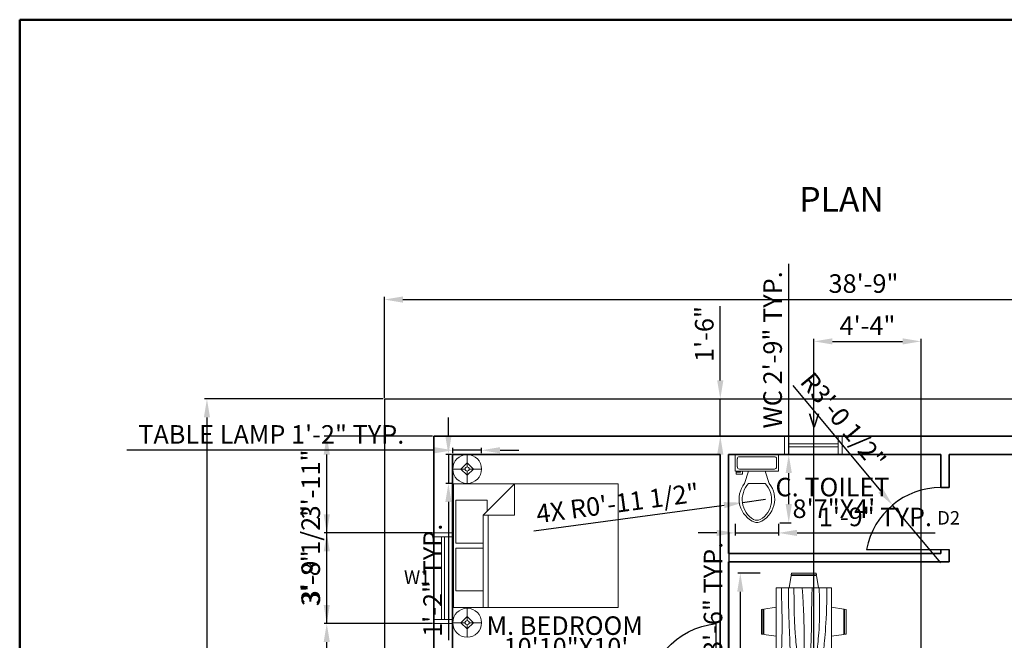
# Model space of a CAD drawing. Units: inches. Extents: x 2113 to 4530, y 1685 to 2353.
# Tile 3 of 6: x 2113 to 2591, y 2052 to 2353. Entities that reach past the tile are written whole.
import ezdxf

# ---------------------------------------------------------------- set-up
doc = ezdxf.new("R2010")
doc.units = ezdxf.units.IN
for name, color, linetype, lineweight in [('A-ANNO-DIMS', 2, 'Continuous', 18), ('A-ANNO-TEXT', 7, 'Continuous', 18), ('A-ANNO-TITL', 7, 'Continuous', 35), ('A-ANNO-TTLB', 7, 'Continuous', 50), ('A-AREA-IDEN', 7, 'Continuous', 18), ('A-DOOR', 3, 'Continuous', 25), ('A-FLOR-FIXT', 9, 'Continuous', 18), ('A-FURN', 8, 'Continuous', 18), ('A-GLAZ', 4, 'Continuous', 18), ('A-WALL', 7, 'Continuous', 35), ('C-PROP', 7, 'Continuous', 25), ('S-ANNO-DIMS', 2, 'Continuous', 18)]:
    doc.layers.add(name, color=color, linetype=linetype, lineweight=lineweight)
doc.styles.get("Standard").update_dxf_attribs({"font": 'arial.ttf'})
doc.dimstyles.new('ISO-25', dxfattribs={"dimtxt": 9, "dimasz": 9, "dimexe": 1.25, "dimexo": 0.625, "dimgap": 2, "dimtad": 1, "dimdec": 1, "dimlunit": 4, "dimtxsty": 'Standard', "dimcen": 2.5, "dimazin": 0, "dimtfac": 1, "dimtdec": 1, "dimtmove": 0, "dimatfit": 3, "dimfxl": 1, "dimarcsym": 0})

# ---------------------------------------------------------------- blocks, each defined once
blk = doc.blocks.new('Dining Set - 36 x 72 in.')
for p, q in [((-22.2343, 26.00059), (-23.4847, 17.99762)), ((-22.2304, 26), (-5.7608, 26)), ((-22, 27.5), (-22.1562, 26.50042)), ((-5.8416, 26.5), (-22.1534, 26.5)), ((-22, 27.5), (-6, 27.5)), ((-5.8437, 26.49966), (-6, 27.5)), ((-4.5152, 17.99762), (-5.7655, 25.99926)), ((5.7657, 26.00059), (4.5153, 17.99762)), ((5.7696, 26), (22.2392, 26)), ((6, 27.5), (5.8438, 26.50042)), ((22.1584, 26.5), (5.8466, 26.5)), ((6, 27.5), (22, 27.5)), ((22.1563, 26.49966), (22, 27.5)), ((23.4848, 17.99762), (22.2345, 25.99926)), ((36, 18), (-36, 18)), ((-36, 18), (-36, -18)), ((36, -18), (36, 18)), ((-45.5, 8), (-44.5004, 8.15617)), ((-45.5, 8), (-45.5, -8)), ((-44.5, -8.15843), (-44.5, 8.15338)), ((-44.0006, 8.23428), (-35.9976, 9.48474)), ((-44, 8.23041), (-44, -8.23915)), ((44.0006, 8.23428), (35.9976, 9.48474)), ((44, 8.23041), (44, -8.23915)), ((44.5, -8.15843), (44.5, 8.15338)), ((45.5, 8), (44.5005, 8.15617)), ((45.5, 8), (45.5, -8)), ((-44.4997, -8.15631), (-45.5, -8)), ((-35.9976, -9.48476), (-43.9993, -8.2345)), ((35.9976, -9.48476), (43.9993, -8.2345)), ((44.4997, -8.15631), (45.5, -8)), ((-36, -18), (36, -18)), ((-22.2343, -26.0006), (-23.4847, -17.99762)), ((-4.5152, -17.99762), (-5.7655, -25.99928)), ((5.7657, -26.0006), (4.5153, -17.99762)), ((23.4848, -17.99762), (22.2345, -25.99928)), ((-22.2304, -26), (-5.7608, -26)), ((-22, -27.5), (-22.1562, -26.50044)), ((-5.8416, -26.5), (-22.1534, -26.5)), ((-22, -27.5), (-6, -27.5)), ((-5.8437, -26.49967), (-6, -27.5)), ((5.7696, -26), (22.2392, -26)), ((6, -27.5), (5.8438, -26.50044)), ((22.1584, -26.5), (5.8466, -26.5)), ((6, -27.5), (22, -27.5)), ((22.1563, -26.49967), (22, -27.5))]:
    blk.add_line(p, q)
for points in [[(-36, 15), (-31.1772, 14.97754), (-26.8079, 14.91406), (-22.8538, 14.81543), (-19.276, 14.6875), (-16.0362, 14.53613), (-13.0957, 14.36718), (-10.4159, 14.18652), (-7.9583, 14), (-5.6904, 13.81315), (-3.6035, 13.63021), (-1.6954, 13.45508), (0.0365, 13.29166), (1.5945, 13.14388), (2.9811, 13.01562), (4.1988, 12.9108), (5.25, 12.83333), (6.1393, 12.78613), (6.8802, 12.76823), (7.4883, 12.77767), (7.9792, 12.8125), (8.3685, 12.87077), (8.6719, 12.95052), (8.9049, 13.0498), (9.0833, 13.16666), (9.2205, 13.29899), (9.3216, 13.44401), (9.3895, 13.59879), (9.4271, 13.76041), (9.4373, 13.92594), (9.4232, 14.09245), (9.3875, 14.257), (9.3333, 14.41666), (9.2638, 14.56917), (9.1836, 14.71484), (9.0975, 14.85465), (9.0104, 14.98958), (8.9272, 15.1206), (8.8529, 15.2487), (8.7922, 15.37483), (8.75, 15.5), (8.7305, 15.62467), (8.7344, 15.74739), (8.7617, 15.86621), (8.8125, 15.97916), (8.8867, 16.08431), (8.9844, 16.17968), (9.1055, 16.26334), (9.25, 16.33333), (9.4189, 16.38802), (9.6172, 16.42708), (9.8506, 16.45052), (10.125, 16.45833), (10.4463, 16.45052), (10.8203, 16.42708), (11.2529, 16.38802), (11.75, 16.33333), (12.3184, 16.26318), (12.9694, 16.17838), (13.7151, 16.07991), (14.5677, 15.96875), (15.5395, 15.84586), (16.6426, 15.71224), (17.8893, 15.56884), (19.2917, 15.41666), (20.859, 15.25667), (22.5879, 15.08984), (24.4721, 14.91715), (26.5052, 14.73958), (28.6809, 14.5581), (30.9929, 14.3737), (33.4347, 14.18733), (36, 14)], [(-36, 10), (-28.9766, 10.14274), (-23.1725, 10.20442), (-18.4241, 10.19775), (-14.5677, 10.13541), (-11.4399, 10.03011), (-8.877, 9.89453), (-6.7154, 9.74137), (-4.7917, 9.58333), (-2.9698, 9.43082), (-1.2246, 9.28515), (0.4415, 9.14534), (2.026, 9.01041), (3.5266, 8.87939), (4.9408, 8.7513), (6.266, 8.62516), (7.5, 8.5), (8.6411, 8.37549), (9.6914, 8.2539), (10.6538, 8.13818), (11.5312, 8.03125), (12.3267, 7.93603), (13.043, 7.85547), (13.6831, 7.79248), (14.25, 7.75), (14.7471, 7.7303), (15.1797, 7.73307), (15.5537, 7.75732), (15.875, 7.80208), (16.1494, 7.86637), (16.3828, 7.94922), (16.5811, 8.04964), (16.75, 8.16666), (16.8944, 8.29915), (17.0143, 8.44531), (17.1089, 8.60319), (17.1771, 8.77083), (17.218, 8.94629), (17.2305, 9.1276), (17.2137, 9.31282), (17.1667, 9.5), (17.0895, 9.6875), (16.987, 9.875), (16.8649, 10.0625), (16.7292, 10.25), (16.5856, 10.4375), (16.4401, 10.625), (16.2985, 10.8125), (16.1667, 11), (16.05, 11.18733), (15.9518, 11.3737), (15.8752, 11.5581), (15.8229, 11.73958), (15.798, 11.91715), (15.8034, 12.08984), (15.842, 12.25667), (15.9167, 12.41666), (16.0295, 12.56836), (16.1784, 12.70833), (16.3605, 12.83268), (16.5729, 12.9375), (16.8127, 13.01888), (17.0768, 13.07291), (17.3625, 13.0957), (17.6667, 13.08333), (17.9894, 13.03312), (18.3418, 12.94726), (18.7382, 12.82918), (19.1927, 12.68229), (19.7195, 12.51001), (20.3327, 12.31575), (21.0465, 12.10294), (21.875, 11.875), (22.8357, 11.63354), (23.959, 11.37304), (25.2786, 11.08618), (26.8282, 10.76562), (28.6414, 10.40405), (30.752, 9.99414), (33.1936, 9.52856), (36, 9)], [(-36, 5.5), (-30.7157, 5.3348), (-26.069, 5.20963), (-21.9946, 5.11767), (-18.4271, 5.05208), (-15.3009, 5.00602), (-12.5508, 4.97265), (-10.1112, 4.94515), (-7.9167, 4.91666), (-5.909, 4.88167), (-4.0586, 4.83984), (-2.3429, 4.79215), (-0.7396, 4.73958), (0.7739, 4.6831), (2.22, 4.6237), (3.6213, 4.56233), (5, 4.5), (6.373, 4.43782), (7.7344, 4.3776), (9.0723, 4.32129), (10.375, 4.27083), (11.6309, 4.22819), (12.8281, 4.19531), (13.9551, 4.17415), (15, 4.16666), (15.954, 4.17448), (16.819, 4.19791), (17.6001, 4.23698), (18.3021, 4.29166), (18.9299, 4.36198), (19.4883, 4.44791), (19.9823, 4.54948), (20.4167, 4.66666), (20.7969, 4.79899), (21.1302, 4.94401), (21.4245, 5.09879), (21.6875, 5.26041), (21.9271, 5.42594), (22.1511, 5.59245), (22.3672, 5.757), (22.5834, 5.91666), (22.8065, 6.06868), (23.0404, 6.21093), (23.2879, 6.34147), (23.5521, 6.45833), (23.8358, 6.55957), (24.142, 6.64323), (24.4735, 6.70735), (24.8334, 6.75), (25.2235, 6.76969), (25.642, 6.76692), (26.0858, 6.74267), (26.5521, 6.69791), (27.0379, 6.63362), (27.5404, 6.55078), (28.0565, 6.45036), (28.5834, 6.33333), (29.1242, 6.19987), (29.7071, 6.04687), (30.3661, 5.87044), (31.1354, 5.66666), (32.0493, 5.43164), (33.142, 5.16146), (34.4475, 4.85221), (36, 4.5)], [(-36, -1), (-30.7915, -0.6591), (-26.0195, -0.38216), (-21.6519, -0.16284), (-17.6563, 0.00521), (-14.0005, 0.12833), (-10.6523, 0.21289), (-7.5796, 0.26522), (-4.75, 0.29166), (-2.134, 0.29793), (0.2878, 0.28711), (2.5317, 0.26163), (4.6146, 0.22396), (6.5529, 0.17651), (8.3633, 0.12174), (10.0623, 0.06209), (11.6667, 0), (13.1899, -0.06201), (14.6341, -0.1211), (15.9982, -0.17432), (17.2813, -0.21875), (18.4823, -0.25147), (19.6003, -0.26953), (20.6343, -0.27002), (21.5834, -0.25), (22.4481, -0.20768), (23.2357, -0.14584), (23.9549, -0.06836), (24.6146, 0.02083), (25.2235, 0.11784), (25.7904, 0.21875), (26.3241, 0.31966), (26.8334, 0.41666), (27.3265, 0.50618), (27.8099, 0.58593), (28.2894, 0.65397), (28.7709, 0.70833), (29.2601, 0.74707), (29.763, 0.76823), (30.2855, 0.76985), (30.8334, 0.75), (31.4088, 0.70784), (31.9994, 0.64713), (32.589, 0.57275), (33.1615, 0.48958), (33.7008, 0.4025), (34.1908, 0.3164), (34.6153, 0.23616), (34.9584, 0.16666), (35.2099, 0.11165), (35.3848, 0.07031), (35.504, 0.04069), (35.5886, 0.02083), (35.6594, 0.00879), (35.7377, 0.0026), (35.8442, 0.00032), (36, 0)], [(-36, -6.5), (-27.1843, -6.31267), (-20.084, -6.1263), (-14.469, -5.9419), (-10.1094, -5.76042), (-6.7752, -5.58285), (-4.2363, -5.41016), (-2.2629, -5.24333), (-0.625, -5.08334), (0.8708, -4.93099), (2.2715, -4.78646), (3.5872, -4.64974), (4.8281, -4.52084), (6.0046, -4.39974), (7.127, -4.28646), (8.2053, -4.18099), (9.25, -4.08334), (10.2705, -3.99382), (11.2734, -3.91407), (12.2647, -3.84603), (13.25, -3.79167), (14.2354, -3.75293), (15.2266, -3.73177), (16.2295, -3.73015), (17.25, -3.75), (18.2912, -3.79248), (19.3451, -3.85547), (20.4009, -3.93604), (21.4479, -4.03125), (22.4754, -4.13819), (23.4727, -4.25391), (24.4289, -4.37549), (25.3334, -4.5), (26.1785, -4.62492), (26.9694, -4.74935), (27.7145, -4.87281), (28.4219, -4.99479), (29.1, -5.11483), (29.7572, -5.23242), (30.4016, -5.34709), (31.0417, -5.45834), (31.6837, -5.56437), (32.3262, -5.65821), (32.9658, -5.73153), (33.599, -5.77604), (34.2224, -5.78345), (34.8327, -5.74545), (35.4264, -5.65373), (36, -5.5)], [(-36, -10), (-26.4022, -9.81299), (-18.4675, -9.62891), (-11.9839, -9.45069), (-6.7396, -9.28125), (-2.5226, -9.12354), (0.8789, -8.98047), (3.6769, -8.85498), (6.0833, -8.75), (8.2767, -8.66765), (10.3021, -8.60677), (12.1712, -8.56543), (13.8958, -8.54167), (15.4876, -8.53353), (16.9583, -8.53907), (18.3197, -8.55632), (19.5834, -8.58334), (20.7616, -8.61841), (21.8685, -8.66081), (22.9188, -8.71004), (23.9271, -8.76563), (24.9081, -8.82707), (25.8763, -8.89388), (26.8465, -8.96558), (27.8334, -9.04167), (28.8474, -9.12118), (29.8828, -9.20117), (30.93, -9.27824), (31.9792, -9.34896), (33.0205, -9.40991), (34.0443, -9.45768), (35.0407, -9.48885), (36, -9.5)], [(-36, -14.5), (-30.0881, -14.33513), (-25.0332, -14.21224), (-20.7312, -14.12647), (-17.0781, -14.07292), (-13.97, -14.04671), (-11.3027, -14.04297), (-8.9724, -14.05681), (-6.875, -14.08334), (-4.9224, -14.11833), (-3.0905, -14.16016), (-1.3709, -14.20785), (0.2448, -14.26042), (1.7647, -14.3169), (3.1973, -14.3763), (4.5507, -14.43767), (5.8333, -14.5), (7.0554, -14.5621), (8.235, -14.62175), (9.3922, -14.67652), (10.5469, -14.72396), (11.7192, -14.76164), (12.929, -14.78711), (14.1965, -14.79794), (15.5417, -14.79167), (16.9933, -14.76424), (18.6152, -14.70508), (20.4804, -14.60197), (22.6615, -14.44271), (25.2312, -14.21509), (28.2624, -13.9069), (31.8277, -13.50594), (36, -13)]]:
    blk.add_lwpolyline(points)
blk = doc.blocks.new('Bed - Queen')
for p, q in [((0, -80.00003), (0, 0)), ((0, 0), (59.99999, 0)), ((59.99999, 0), (59.99999, -80.00003)), ((7.99999, -1.2), (28.79998, -1.2)), ((7.99999, -14.4), (7.99999, -1.2)), ((28.79998, -1.2), (28.79998, -14.4)), ((31.19999, -1.2), (51.99999, -1.2)), ((31.19999, -14.4), (31.19999, -1.2)), ((51.99999, -1.2), (51.99999, -16.4)), ((0, -14.4), (44.8, -14.4)), ((44.8, -16.8), (0, -16.8)), ((59.99999, -29.6), (44.8, -14.4)), ((44.8, -14.4), (44.8, -29.6)), ((51.99999, -16.4), (46.79936, -16.4)), ((44.8, -29.6), (59.99999, -29.6)), ((59.99999, -80.00003), (0, -80.00003))]:
    blk.add_line(p, q)
blk = doc.blocks.new('Lamp - Table')
for p, q in [((0, 7), (0, 1)), ((-1, 0), (-7, 0)), ((0, 3), (-3, 0)), ((-3, 0), (0, -3)), ((3, 0), (0, 3)), ((0, -3), (3, 0)), ((1, 0), (7, 0)), ((0, -1), (0, -7))]:
    blk.add_line(p, q)
for radius in [7, 1]:
    blk.add_circle((0, 0), radius)
blk = doc.blocks.new('Toilet - top')
for p, q in [((9.5, -6), (9.5, -2)), ((-10, -8.5), (-8, -8.5)), ((-10, -9.5), (-10, -8.5)), ((-7, -9.5), (-10, -9.5)), ((-8, -8.5), (-8, -8)), ((-7, -8), (-7, -9.5)), ((-4, -8), (-6, -14)), ((4, -8), (6, -14)), ((4, -14), (-4, -14))]:
    blk.add_line(p, q)
blk.add_lwpolyline([(10.5, -8), (10.5, 0), (-10.5, 0), (-10.5, -8)], close=True)
for points in [[(-9.5, -2), (-9.5, -6)], [(8.5, -1), (-8.5, -1)], [(-8.5, -7), (8.5, -7)]]:
    blk.add_lwpolyline(points)
for centre, radius, start, end in [((-8.62, -1.88), 0.884, 81.8699, 188.1301), ((8.62, -1.88), 0.884, 351.8699, 98.1301), ((-8.62, -6.12), 0.884, 171.8699, 278.1301), ((8.62, -6.12), 0.884, 261.8699, 8.1301), ((3.52, -21.58), 12.17, 141.4691, 247.9714), ((4.2, -21.82), 11.33, 136.3677, 238.9468), ((-3.52, -21.58), 12.17, 292.0284, 38.5307), ((-4.2, -21.82), 11.33, 301.053, 43.6321), ((0, -27.88), 4, 245.7318, 294.2682), ((0, -29), 4, 254.8605, 285.1395)]:
    blk.add_arc(centre, radius, start, end)
blk = doc.blocks.new('*D7')
at = {"layer": 'A-ANNO-DIMS', "color": 0, "lineweight": -2, "transparency": 16777216}
for p, q in [((2289.73, 2169.51), (2289.73, 2218.38)), ((2298.73, 2217.13), (2745.73, 2217.13)), ((2754.73, 2169.51), (2754.73, 2218.38))]:
    blk.add_line(p, q, dxfattribs=at)
at = {"layer": 'A-ANNO-DIMS', "color": 0, "transparency": 16777216}
for points in [[(2298.73, 2218.63), (2298.73, 2215.63), (2289.73, 2217.13)], [(2745.73, 2218.63), (2745.73, 2215.63), (2754.73, 2217.13)]]:
    blk.add_solid(points, dxfattribs=at)
at = {"layer": 'Defpoints', "color": 0, "transparency": 16777216}
for p in [(2754.73, 2217.13), (2289.73, 2168.89), (2754.73, 2168.89)]:
    blk.add_point(p, dxfattribs=at)
at = {"layer": 'A-ANNO-DIMS', "color": 0, "transparency": 16777216, "insert": (2522.23, 2223.73), "char_height": 9, "attachment_point": 5}
blk.add_mtext('38\'-9"', dxfattribs=at)
blk = doc.blocks.new('*D8')
at = {"layer": 'A-ANNO-DIMS', "color": 0, "lineweight": -2, "transparency": 16777216}
for p, q in [((2289.11, 2168.89), (2202.39, 2168.89)), ((2203.64, 2159.89), (2203.64, 1781.89)), ((2289.11, 1772.89), (2202.39, 1772.89))]:
    blk.add_line(p, q, dxfattribs=at)
at = {"layer": 'A-ANNO-DIMS', "color": 0, "transparency": 16777216}
for points in [[(2202.14, 2159.89), (2205.14, 2159.89), (2203.64, 2168.89)], [(2202.14, 1781.89), (2205.14, 1781.89), (2203.64, 1772.89)]]:
    blk.add_solid(points, dxfattribs=at)
at = {"layer": 'Defpoints', "color": 0, "transparency": 16777216}
for p in [(2289.73, 2168.89), (2203.64, 1772.89), (2289.73, 1772.89)]:
    blk.add_point(p, dxfattribs=at)
at = {"layer": 'A-ANNO-DIMS', "color": 0, "transparency": 16777216, "insert": (2197.04, 1970.89), "char_height": 9, "attachment_point": 5, "rotation": 90}
blk.add_mtext("33'", dxfattribs=at)
blk = doc.blocks.new('*D28')
at = {"layer": 'A-ANNO-DIMS', "color": 0, "lineweight": -2, "transparency": 16777216}
for p, q in [((2452.73, 2177.89), (2452.73, 2213.96)), ((2290.36, 2168.89), (2453.98, 2168.89)), ((2452.73, 2150.89), (2452.73, 2168.89)), ((2314.36, 2150.89), (2453.98, 2150.89)), ((2452.73, 2141.89), (2452.73, 2132.89))]:
    blk.add_line(p, q, dxfattribs=at)
at = {"layer": 'A-ANNO-DIMS', "color": 0, "transparency": 16777216}
for points in [[(2451.23, 2177.89), (2454.23, 2177.89), (2452.73, 2168.89)], [(2451.23, 2141.89), (2454.23, 2141.89), (2452.73, 2150.89)]]:
    blk.add_solid(points, dxfattribs=at)
at = {"layer": 'Defpoints', "color": 0, "transparency": 16777216}
for p in [(2289.73, 2168.89), (2452.73, 2168.89), (2313.73, 2150.89)]:
    blk.add_point(p, dxfattribs=at)
at = {"layer": 'A-ANNO-DIMS', "color": 0, "transparency": 16777216, "insert": (2446.14, 2200.42), "char_height": 9, "attachment_point": 5, "rotation": 90}
blk.add_mtext('1\'-6"', dxfattribs=at)
blk = doc.blocks.new('*D29')
at = {"layer": 'A-ANNO-DIMS', "color": 0, "lineweight": -2, "transparency": 16777216}
for p, q in [((2289.73, 2168.26), (2289.73, 1969.64)), ((2313.73, 2150.26), (2313.73, 1969.64)), ((2304.73, 1970.89), (2298.73, 1970.89))]:
    blk.add_line(p, q, dxfattribs=at)
at = {"layer": 'A-ANNO-DIMS', "color": 0, "transparency": 16777216}
for points in [[(2298.73, 1972.39), (2298.73, 1969.39), (2289.73, 1970.89)], [(2304.73, 1972.39), (2304.73, 1969.39), (2313.73, 1970.89)]]:
    blk.add_solid(points, dxfattribs=at)
at = {"layer": 'Defpoints', "color": 0, "transparency": 16777216}
for p in [(2289.73, 2168.89), (2313.73, 2150.89), (2289.73, 1970.89)]:
    blk.add_point(p, dxfattribs=at)
at = {"layer": 'A-ANNO-DIMS', "color": 0, "transparency": 16777216, "insert": (2301.73, 1977.4), "char_height": 9, "attachment_point": 5}
blk.add_mtext("2'", dxfattribs=at)
blk = doc.blocks.new('DOOR-D1-SWING')
blk.add_line((34, 42), (34, 0))
blk.add_arc((38.24, 38), 38.24, 180, 263.6403)
blk = doc.blocks.new('LOT-465X396')
for p, q in [((0, 396), (465, 396)), ((0, 396), (0, 0)), ((465, 396), (465, 0)), ((0, 0), (465, 0))]:
    blk.add_line(p, q)
blk = doc.blocks.new('*D42')
at = {"layer": 'Defpoints', "color": 0, "transparency": 16777216}
for p in [(2322.91, 2143.99), (2322.91, 2141.89), (2336.91, 2141.89)]:
    blk.add_point(p, dxfattribs=at)
at = {"layer": 'S-ANNO-DIMS', "color": 0, "lineweight": -2, "transparency": 16777216}
for p, q in [((2313.91, 2143.99), (2164.76, 2143.99)), ((2322.91, 2142.51), (2322.91, 2145.24)), ((2336.91, 2143.99), (2322.91, 2143.99)), ((2336.91, 2142.51), (2336.91, 2145.24)), ((2345.91, 2143.99), (2354.91, 2143.99))]:
    blk.add_line(p, q, dxfattribs=at)
at = {"layer": 'S-ANNO-DIMS', "color": 0, "transparency": 16777216}
for points in [[(2313.91, 2145.49), (2313.91, 2142.49), (2322.91, 2143.99)], [(2345.91, 2145.49), (2345.91, 2142.49), (2336.91, 2143.99)]]:
    blk.add_solid(points, dxfattribs=at)
at = {"layer": 'S-ANNO-DIMS', "color": 0, "transparency": 16777216, "insert": (2234.84, 2150.51), "char_height": 9, "attachment_point": 5}
blk.add_mtext('TABLE LAMP 1\'-2" TYP.', dxfattribs=at)
blk = doc.blocks.new('*D43')
at = {"layer": 'Defpoints', "color": 0, "transparency": 16777216}
for p in [(2322.91, 2141.89), (2320.81, 2127.89), (2322.91, 2127.89)]:
    blk.add_point(p, dxfattribs=at)
at = {"layer": 'S-ANNO-DIMS', "color": 0, "lineweight": -2, "transparency": 16777216}
for p, q in [((2320.81, 2150.89), (2320.81, 2159.89)), ((2322.28, 2141.89), (2319.56, 2141.89)), ((2320.81, 2141.89), (2320.81, 2127.89)), ((2322.28, 2127.89), (2319.56, 2127.89)), ((2320.81, 2118.89), (2320.81, 2051.87))]:
    blk.add_line(p, q, dxfattribs=at)
at = {"layer": 'S-ANNO-DIMS', "color": 0, "transparency": 16777216}
for points in [[(2319.31, 2150.89), (2322.31, 2150.89), (2320.81, 2141.89)], [(2319.31, 2118.89), (2322.31, 2118.89), (2320.81, 2127.89)]]:
    blk.add_solid(points, dxfattribs=at)
at = {"layer": 'S-ANNO-DIMS', "color": 0, "transparency": 16777216, "insert": (2314.29, 2080.88), "char_height": 9, "attachment_point": 5, "rotation": 90}
blk.add_mtext('1\'-2" TYP.', dxfattribs=at)
blk = doc.blocks.new('*D52')
at = {"layer": 'Defpoints', "color": 0, "transparency": 16777216}
for p in [(2481.01, 2141.87), (2485.96, 2141.87), (2481.01, 2108.83)]:
    blk.add_point(p, dxfattribs=at)
at = {"layer": 'S-ANNO-DIMS', "color": 0, "lineweight": -2, "transparency": 16777216}
for p, q in [((2485.96, 2141.87), (2485.96, 2234.54)), ((2481.63, 2141.87), (2487.21, 2141.87)), ((2485.96, 2117.83), (2485.96, 2132.87)), ((2481.63, 2108.83), (2487.21, 2108.83))]:
    blk.add_line(p, q, dxfattribs=at)
at = {"layer": 'S-ANNO-DIMS', "color": 0, "transparency": 16777216}
for points in [[(2484.46, 2132.87), (2487.46, 2132.87), (2485.96, 2141.87)], [(2484.46, 2117.83), (2487.46, 2117.83), (2485.96, 2108.83)]]:
    blk.add_solid(points, dxfattribs=at)
at = {"layer": 'S-ANNO-DIMS', "color": 0, "transparency": 16777216, "insert": (2479.31, 2192.71), "char_height": 9, "attachment_point": 5, "rotation": 90}
blk.add_mtext('WC 2\'-9" TYP.', dxfattribs=at)
blk = doc.blocks.new('*D53')
at = {"layer": 'Defpoints', "color": 0, "transparency": 16777216}
for p in [(2460.01, 2108.83), (2481.01, 2108.83), (2481.01, 2103.87)]:
    blk.add_point(p, dxfattribs=at)
at = {"layer": 'S-ANNO-DIMS', "color": 0, "lineweight": -2, "transparency": 16777216}
for p, q in [((2460.01, 2108.2), (2460.01, 2102.62)), ((2481.01, 2108.2), (2481.01, 2102.62)), ((2451.01, 2103.87), (2442.01, 2103.87)), ((2460.01, 2103.87), (2481.01, 2103.87)), ((2490.01, 2103.87), (2557.02, 2103.87))]:
    blk.add_line(p, q, dxfattribs=at)
at = {"layer": 'S-ANNO-DIMS', "color": 0, "transparency": 16777216}
for points in [[(2451.01, 2105.37), (2451.01, 2102.37), (2460.01, 2103.87)], [(2490.01, 2105.37), (2490.01, 2102.37), (2481.01, 2103.87)]]:
    blk.add_solid(points, dxfattribs=at)
at = {"layer": 'S-ANNO-DIMS', "color": 0, "transparency": 16777216, "insert": (2528.01, 2110.46), "char_height": 9, "attachment_point": 5}
blk.add_mtext('1\'-9" TYP.', dxfattribs=at)
blk = doc.blocks.new('*D54')
at = {"layer": 'Defpoints', "color": 0, "transparency": 16777216}
for p in [(2450.73, 1975.89), (2457.03, 1975.89), (2450.73, 1933.89)]:
    blk.add_point(p, dxfattribs=at)
at = {"layer": 'S-ANNO-DIMS', "color": 0, "lineweight": -2, "transparency": 16777216}
for p, q in [((2457.03, 1975.89), (2457.03, 2104.07)), ((2451.36, 1975.89), (2458.28, 1975.89)), ((2457.03, 1942.89), (2457.03, 1966.89)), ((2451.36, 1933.89), (2458.28, 1933.89))]:
    blk.add_line(p, q, dxfattribs=at)
at = {"layer": 'S-ANNO-DIMS', "color": 0, "transparency": 16777216}
for points in [[(2455.53, 1966.89), (2458.53, 1966.89), (2457.03, 1975.89)], [(2455.53, 1942.89), (2458.53, 1942.89), (2457.03, 1933.89)]]:
    blk.add_solid(points, dxfattribs=at)
at = {"layer": 'S-ANNO-DIMS', "color": 0, "transparency": 16777216, "insert": (2450.37, 2044.48), "char_height": 9, "attachment_point": 5, "rotation": 90}
blk.add_mtext('DOOR D1 3\'-6" TYP.', dxfattribs=at)
blk = doc.blocks.new('*D58')
at = {"layer": 'Defpoints', "color": 0, "transparency": 16777216}
for p in [(2472.67, 2084.34), (2462.46, 2016.25), (2472.67, 2016.25)]:
    blk.add_point(p, dxfattribs=at)
at = {"layer": 'S-ANNO-DIMS', "color": 0, "lineweight": -2, "transparency": 16777216}
for p, q in [((2472.05, 2084.34), (2461.21, 2084.34)), ((2462.46, 2075.34), (2462.46, 2025.25)), ((2472.05, 2016.25), (2461.21, 2016.25)), ((2462.46, 2016.25), (2462.46, 1904.33))]:
    blk.add_line(p, q, dxfattribs=at)
at = {"layer": 'S-ANNO-DIMS', "color": 0, "transparency": 16777216}
for points in [[(2460.96, 2075.34), (2463.96, 2075.34), (2462.46, 2084.34)], [(2460.96, 2025.25), (2463.96, 2025.25), (2462.46, 2016.25)]]:
    blk.add_solid(points, dxfattribs=at)
at = {"layer": 'S-ANNO-DIMS', "color": 0, "transparency": 16777216, "insert": (2455.81, 1955.79), "char_height": 9, "attachment_point": 5, "rotation": 90}
blk.add_mtext('DINING SET 5\'-8"', dxfattribs=at)
blk = doc.blocks.new('*D93')
at = {"layer": 'Defpoints', "color": 0, "transparency": 16777216}
for p in [(2550.184017, 2196.835797), (2498.184017, 1863.885797), (2550.184017, 1863.885797)]:
    blk.add_point(p, dxfattribs=at)
at = {"layer": 'S-ANNO-DIMS', "color": 0, "lineweight": -2, "transparency": 16777216}
for p, q in [((2498.184017, 1864.510797), (2498.184017, 2198.085797)), ((2550.184017, 1864.510797), (2550.184017, 2198.085797)), ((2507.184017, 2196.835797), (2541.184017, 2196.835797))]:
    blk.add_line(p, q, dxfattribs=at)
at = {"layer": 'S-ANNO-DIMS', "color": 0, "transparency": 16777216}
for points in [[(2507.184017, 2198.335797), (2507.184017, 2195.335797), (2498.184017, 2196.835797)], [(2541.184017, 2198.335797), (2541.184017, 2195.335797), (2550.184017, 2196.835797)]]:
    blk.add_solid(points, dxfattribs=at)
at = {"layer": 'S-ANNO-DIMS', "color": 0, "transparency": 16777216, "insert": (2524.184017, 2203.335797), "char_height": 9, "attachment_point": 5}
blk.add_mtext('4\'-4"', dxfattribs=at)
blk = doc.blocks.new('*D98')
at = {"layer": 'Defpoints', "color": 0, "transparency": 16777216}
for p in [(2261.78, 2059.89), (2313.73, 2059.89), (2313.73, 2014.53)]:
    blk.add_point(p, dxfattribs=at)
at = {"layer": 'S-ANNO-DIMS', "color": 0, "lineweight": -2, "transparency": 16777216}
for p, q in [((2261.78, 2059.89), (2261.78, 2117.78)), ((2313.11, 2059.89), (2260.53, 2059.89)), ((2261.78, 2023.53), (2261.78, 2050.89)), ((2313.11, 2014.53), (2260.53, 2014.53))]:
    blk.add_line(p, q, dxfattribs=at)
at = {"layer": 'S-ANNO-DIMS', "color": 0, "transparency": 16777216}
for points in [[(2260.28, 2050.89), (2263.28, 2050.89), (2261.78, 2059.89)], [(2260.28, 2023.53), (2263.28, 2023.53), (2261.78, 2014.53)]]:
    blk.add_solid(points, dxfattribs=at)
at = {"layer": 'S-ANNO-DIMS', "color": 0, "transparency": 16777216, "insert": (2255.13, 2093.33), "char_height": 9, "attachment_point": 5, "rotation": 90}
blk.add_mtext('3\'-9 1/2"', dxfattribs=at)
blk = doc.blocks.new('*D99')
at = {"layer": 'Defpoints', "color": 0, "transparency": 16777216}
for p in [(2261.78, 2103.89), (2313.73, 2103.89), (2313.73, 2059.89)]:
    blk.add_point(p, dxfattribs=at)
at = {"layer": 'S-ANNO-DIMS', "color": 0, "lineweight": -2, "transparency": 16777216}
for p, q in [((2313.11, 2103.89), (2260.53, 2103.89)), ((2261.78, 2068.89), (2261.78, 2094.89)), ((2313.11, 2059.89), (2260.53, 2059.89))]:
    blk.add_line(p, q, dxfattribs=at)
at = {"layer": 'S-ANNO-DIMS', "color": 0, "transparency": 16777216}
for points in [[(2260.28, 2094.89), (2263.28, 2094.89), (2261.78, 2103.89)], [(2260.28, 2068.89), (2263.28, 2068.89), (2261.78, 2059.89)]]:
    blk.add_solid(points, dxfattribs=at)
at = {"layer": 'S-ANNO-DIMS', "color": 0, "transparency": 16777216, "insert": (2255.18, 2081.89), "char_height": 9, "attachment_point": 5, "rotation": 90}
blk.add_mtext('3\'-8"', dxfattribs=at)
blk = doc.blocks.new('*D100')
at = {"layer": 'Defpoints', "color": 0, "transparency": 16777216}
for p in [(2261.78, 2150.89), (2313.73, 2150.89), (2313.73, 2103.89)]:
    blk.add_point(p, dxfattribs=at)
at = {"layer": 'S-ANNO-DIMS', "color": 0, "lineweight": -2, "transparency": 16777216}
for p, q in [((2313.11, 2150.89), (2260.53, 2150.89)), ((2261.78, 2112.89), (2261.78, 2141.89)), ((2313.11, 2103.89), (2260.53, 2103.89))]:
    blk.add_line(p, q, dxfattribs=at)
at = {"layer": 'S-ANNO-DIMS', "color": 0, "transparency": 16777216}
for points in [[(2260.28, 2141.89), (2263.28, 2141.89), (2261.78, 2150.89)], [(2260.28, 2112.89), (2263.28, 2112.89), (2261.78, 2103.89)]]:
    blk.add_solid(points, dxfattribs=at)
at = {"layer": 'S-ANNO-DIMS', "color": 0, "transparency": 16777216, "insert": (2255.18, 2127.39), "char_height": 9, "attachment_point": 5, "rotation": 90}
blk.add_mtext('3\'-11"', dxfattribs=at)
blk = doc.blocks.new('*D105')
at = {"layer": 'Defpoints', "color": 0, "transparency": 16777216}
for p in [(2536.3, 2117.4), (2559.73, 2089.29)]:
    blk.add_point(p, dxfattribs=at)
at = {"layer": 'S-ANNO-DIMS', "color": 0, "lineweight": -2, "transparency": 16777216}
for p, q in [((2487.96, 2175.41), (2530.54, 2124.32)), ((2559.73, 2089.29), (2536.3, 2117.4))]:
    blk.add_line(p, q, dxfattribs=at)
at = {"layer": 'S-ANNO-DIMS', "color": 0, "transparency": 16777216}
blk.add_solid([(2531.69, 2125.28), (2529.39, 2123.36), (2536.3, 2117.4)], dxfattribs=at)
at = {"layer": 'S-ANNO-DIMS', "color": 0, "transparency": 16777216, "insert": (2511.48, 2157.58), "char_height": 9, "attachment_point": 5, "rotation": 309.8048}
blk.add_mtext('R3\'-0 1/2"', dxfattribs=at)
blk = doc.blocks.new('*D109')
at = {"layer": 'Defpoints', "color": 0, "transparency": 16777216}
for p in [(2463.48, 2118.54), (2474.71, 2120.05)]:
    blk.add_point(p, dxfattribs=at)
at = {"layer": 'S-ANNO-DIMS', "color": 0, "lineweight": -2, "transparency": 16777216}
for p, q in [((2362.19, 2104.93), (2454.56, 2117.35)), ((2474.71, 2120.05), (2463.48, 2118.54))]:
    blk.add_line(p, q, dxfattribs=at)
at = {"layer": 'S-ANNO-DIMS', "color": 0, "transparency": 16777216}
blk.add_solid([(2454.36, 2118.83), (2454.76, 2115.86), (2463.48, 2118.54)], dxfattribs=at)
at = {"layer": 'S-ANNO-DIMS', "color": 0, "transparency": 16777216, "insert": (2403.03, 2117.13), "char_height": 9, "attachment_point": 5, "rotation": 7.6571}
blk.add_mtext('4X R0\'-11 1/2"', dxfattribs=at)

msp = doc.modelspace()

# ---------------------------------------------------------------- linework, layer by layer
at = {"layer": 'A-ANNO-TTLB'}
msp.add_lwpolyline([(2112.77, 2352.97), (4498.42, 2352.97), (4498.42, 1685.12), (2112.77, 1685.12)], close=True, dxfattribs=at)
at = {"layer": 'A-DOOR'}
msp.add_line((2523.73, 2095.89), (2563.73, 2095.89), dxfattribs=at)
msp.add_arc((2559.73, 2089.29), 36.6, 90, 169.6111, dxfattribs=at)
at = {"layer": 'A-GLAZ'}
for p, q in [((2483.94, 2150.89), (2483.94, 2141.89)), ((2485.94, 2150.89), (2485.94, 2141.89)), ((2509.94, 2150.89), (2509.94, 2141.89)), ((2511.94, 2150.89), (2511.94, 2141.89)), ((2509.94, 2147.14), (2485.94, 2147.14)), ((2509.94, 2145.64), (2485.94, 2145.64)), ((2313.73, 2103.89), (2322.73, 2103.89)), ((2313.73, 2101.89), (2322.73, 2101.89)), ((2317.45, 2061.89), (2317.45, 2101.89)), ((2318.95, 2061.89), (2318.95, 2101.89)), ((2313.73, 2061.89), (2322.73, 2061.89)), ((2313.73, 2059.89), (2322.73, 2059.89))]:
    msp.add_line(p, q, dxfattribs=at)
at = {"layer": 'A-WALL'}
for p, q in [((2313.73, 2150.89), (2730.73, 2150.89)), ((2313.73, 2150.89), (2313.73, 1772.89)), ((2322.73, 2141.89), (2322.73, 2021.89)), ((2322.73, 2141.89), (2452.73, 2141.89)), ((2452.73, 2141.89), (2452.73, 2021.89)), ((2456.73, 2141.89), (2456.73, 2093.89)), ((2456.73, 2141.89), (2559.73, 2141.89)), ((2559.73, 2141.89), (2559.73, 2125.89)), ((2563.73, 2141.89), (2563.73, 2125.89)), ((2563.73, 2141.89), (2601.73, 2141.89)), ((2559.73, 2125.89), (2563.73, 2125.89)), ((2456.73, 2093.89), (2559.73, 2093.89)), ((2559.73, 2095.89), (2559.73, 2093.89)), ((2563.73, 2095.89), (2563.73, 2089.89)), ((2456.73, 2089.89), (2563.73, 2089.89)), ((2456.73, 2089.89), (2456.73, 2017.89))]:
    msp.add_line(p, q, dxfattribs=at)

# ---------------------------------------------------------------- block references
at = {"layer": 'A-DOOR', "extrusion": (0, 0, -1), "zscale": -1, "rotation": 180}
msp.add_blockref('DOOR-D1-SWING', (-2416.73, 2059.89), dxfattribs=at)
at = {"layer": 'A-FLOR-FIXT'}
msp.add_blockref('Toilet - top', (2470.51, 2141.87), dxfattribs=at)
at = {"layer": 'A-FURN'}
for name, p, rotation in [('Lamp - Table', (2329.91, 2134.89), 180), ('Bed - Queen', (2323.25, 2067.71), 90), ('Lamp - Table', (2329.91, 2060.28), 180)]:
    msp.add_blockref(name, p, dxfattribs=dict(at, rotation=rotation))
at = {"layer": 'A-FURN', "xscale": 0.7483003964013882, "yscale": 0.7483003964013882, "zscale": 0.7483003964013882, "rotation": 269.9999999999999}
msp.add_blockref('Dining Set - 36 x 72 in.', (2493.25, 2050.3), dxfattribs=at)
at = {"layer": 'C-PROP'}
msp.add_blockref('LOT-465X396', (2289.73, 1772.89), dxfattribs=at)

# ---------------------------------------------------------------- texts
at = {"layer": 'A-ANNO-TEXT'}
for s, p in [('V', (2495.66, 2155.16)), (' D2', (2556.01, 2107.92)), ('W1', (2299.26, 2079.09))]:
    msp.add_text(s, height=6.54, dxfattribs=at).set_placement(p)
at = {"layer": 'A-ANNO-TITL'}
msp.add_text('       PLAN', height=12, dxfattribs=at).set_placement((2465.39, 2259.78))
at = {"layer": 'A-AREA-IDEN'}
for s, p in [('C. TOILET', (2479.55, 2121.61)), ('   8\'7"X4\'', (2479.55, 2111.11)), ('M. BEDROOM', (2339.3, 2054.37)), ('   10\'10"X10\'', (2339.3, 2043.86))]:
    msp.add_text(s, height=9, dxfattribs=at).set_placement(p)

# ---------------------------------------------------------------- dimensions: what is measured, and where the dimension line sits
at = {"layer": 'A-ANNO-DIMS'}
for base, p1, p2, picture, middle in [((2754.73, 2217.13), (2289.73, 2168.89), (2754.73, 2168.89), '*D7', (2522.23, 2223.73)), ((2289.73, 1970.89), (2313.73, 2150.89), (2289.73, 2168.89), '*D29', (2301.73, 1977.4))]:
    dim = msp.add_linear_dim(base=base, p1=p1, p2=p2, dimstyle='ISO-25', override={"dimclrd": 0, "dimclre": 0, "dimclrt": 0}, dxfattribs=at)
    dim.commit()
    dim.dimension.update_dxf_attribs({"geometry": picture, "text_midpoint": middle})
for base, p1, p2, picture, middle in [((2452.73, 2168.89), (2313.73, 2150.89), (2289.73, 2168.89), '*D28', (2446.14, 2200.42)), ((2203.64, 1772.89), (2289.73, 2168.89), (2289.73, 1772.89), '*D8', (2197.04, 1970.89))]:
    dim = msp.add_linear_dim(base=base, p1=p1, p2=p2, angle=90, dimstyle='ISO-25', override={"dimclrd": 0, "dimclre": 0, "dimclrt": 0}, dxfattribs=at)
    dim.commit()
    dim.dimension.update_dxf_attribs({"geometry": picture, "text_midpoint": middle})
at = {"layer": 'S-ANNO-DIMS'}
for base, p1, p2, angle, text, picture, middle in [((2485.96, 2141.87), (2481.01, 2108.83), (2481.01, 2141.87), 90, 'WC <> TYP.', '*D52', (2479.31, 2192.71)), ((2322.91, 2143.99), (2336.91, 2141.89), (2322.91, 2141.89), 180, 'TABLE LAMP <> TYP.', '*D42', (2234.84, 2150.51)), ((2320.81, 2127.89), (2322.91, 2141.89), (2322.91, 2127.89), 270, '<> TYP.', '*D43', (2314.29, 2080.88)), ((2457.03, 1975.89), (2450.73, 1933.89), (2450.73, 1975.89), 90, 'DOOR D1 <> TYP.', '*D54', (2450.37, 2044.48)), ((2462.46, 2016.25), (2472.67, 2084.34), (2472.67, 2016.25), 270, 'DINING SET <>', '*D58', (2455.81, 1955.79))]:
    dim = msp.add_linear_dim(base=base, p1=p1, p2=p2, angle=angle, text=text, dimstyle='ISO-25', override={"dimdec": 1, "dimlfac": 1, "dimrnd": 0, "dimzin": 1, "dimdsep": 46, "dimlunit": 4, "dimfrac": 2}, dxfattribs=at)
    dim.commit()
    dim.dimension.update_dxf_attribs({"geometry": picture, "text_midpoint": middle})
dim = msp.add_linear_dim(base=(2550.18, 2196.84), p1=(2498.18, 1863.89), p2=(2550.18, 1863.89), dimstyle='ISO-25', override={"dimdec": 1, "dimlfac": 1, "dimrnd": 0, "dimzin": 1, "dimdsep": 46, "dimlunit": 4, "dimfrac": 2}, dxfattribs=at)
dim.commit()
dim.dimension.update_dxf_attribs({"geometry": '*D93', "text_midpoint": (2524.18, 2203.34)})
dim = msp.add_radius_dim(center=(2559.73, 2089.29), mpoint=(2536.3, 2117.4), dimstyle='ISO-25', override={"dimdec": 1, "dimlfac": 1, "dimrnd": 0, "dimzin": 1, "dimdsep": 46, "dimlunit": 4, "dimfrac": 2}, dxfattribs=at)
dim.commit()
dim.dimension.update_dxf_attribs({"geometry": '*D105', "text_midpoint": (2511.48, 2157.58)})
for base, p1, p2, picture, middle in [((2261.78, 2150.89), (2313.73, 2103.89), (2313.73, 2150.89), '*D100', (2255.18, 2127.39)), ((2261.78, 2059.89), (2313.73, 2014.53), (2313.73, 2059.89), '*D98', (2255.13, 2093.33)), ((2261.78, 2103.89), (2313.73, 2059.89), (2313.73, 2103.89), '*D99', (2255.18, 2081.89))]:
    dim = msp.add_linear_dim(base=base, p1=p1, p2=p2, angle=90, dimstyle='ISO-25', override={"dimdec": 1, "dimlfac": 1, "dimrnd": 0, "dimzin": 1, "dimdsep": 46, "dimlunit": 4, "dimfrac": 2}, dxfattribs=at)
    dim.commit()
    dim.dimension.update_dxf_attribs({"geometry": picture, "text_midpoint": middle})
dim = msp.add_radius_dim(center=(2474.71, 2120.05), mpoint=(2463.48, 2118.54), text='4X <>', dimstyle='ISO-25', override={"dimdec": 1, "dimlfac": 1, "dimrnd": 0, "dimzin": 1, "dimdsep": 46, "dimlunit": 4, "dimfrac": 2}, dxfattribs=at)
dim.commit()
dim.dimension.update_dxf_attribs({"geometry": '*D109', "text_midpoint": (2403.03, 2117.13)})
dim = msp.add_linear_dim(base=(2481.01, 2103.87), p1=(2460.01, 2108.83), p2=(2481.01, 2108.83), text='<> TYP.', dimstyle='ISO-25', override={"dimdec": 1, "dimlfac": 1, "dimrnd": 0, "dimzin": 1, "dimdsep": 46, "dimlunit": 4, "dimfrac": 2}, dxfattribs=at)
dim.commit()
dim.dimension.update_dxf_attribs({"geometry": '*D53', "text_midpoint": (2528.01, 2110.46)})

doc.saveas('drawing.dxf')
